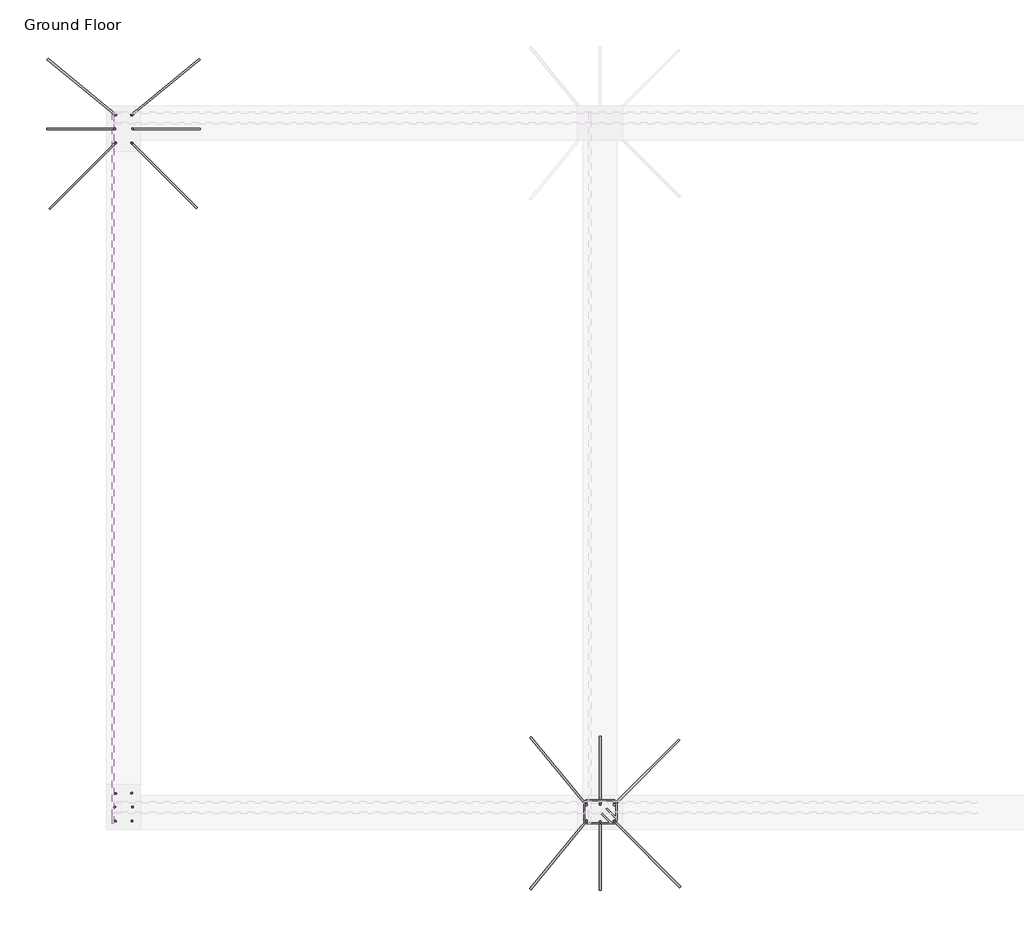
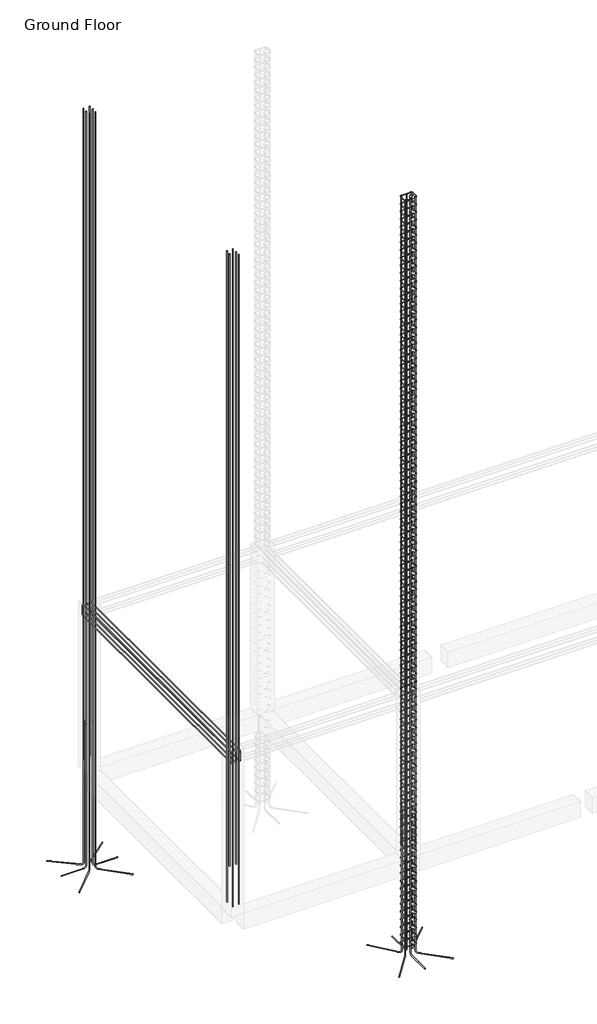
# One storey, part 2 of 5: 33 reinforcing bars.
"""IFC4 building model written with IfcOpenShell, lengths in millimetres."""

from ifc_helpers import new_model, si_unit, point, frame, origin, place, context, project, spatial, polyline, circle_curve, trimmed, segment, composite_curve, source, transform, mapped, element, save
from ifc_brep_helpers import swept_disk

model = new_model("IFC4")

# Units and contexts
model_context = context("Model", 3, world=origin())
ifc_project = project(units=[si_unit("LENGTHUNIT", "METRE", prefix="MILLI")], contexts=[model_context])

# Site, building, storey
site = spatial("IfcSite", under=ifc_project)
building = spatial("IfcBuilding", under=site)
storey = spatial("IfcBuildingStorey", under=building, Name="Ground Floor", Elevation=0.0)

# Reinforcing bars
placement = place(None, origin())
element("IfcReinforcingBar", 1, at=placement, inside=storey, context=model_context, shape_type="SolidModel", body=[
    swept_disk(composite_curve([segment(polyline([(-9208.3090827, 245.2834631, 12794.2305276), (-9208.3090827, 245.2834631, 171.0746196)]), True, "CONTINUOUS")], self_intersect=False), 6.0),
])
element("IfcReinforcingBar", 2, at=placement, inside=storey, context=model_context, shape_type="SolidModel", body=[
    swept_disk(composite_curve([segment(polyline([(-9204.3117524, 339.6230123, 888.7528218), (-9204.3117524, 339.6230123, 12792.7935546)]), True, "CONTINUOUS")], self_intersect=False), 6.0),
])
element("IfcReinforcingBar", 3, at=placement, inside=storey, context=model_context, shape_type="SolidModel", body=[
    swept_disk(composite_curve([segment(polyline([(-9210.4117524, 433.7797002, 12790.6127039), (-9210.4117524, 433.7797002, 154.6015232)]), True, "CONTINUOUS")], self_intersect=False), 6.0),
])
element("IfcReinforcingBar", 4, at=placement, inside=storey, context=model_context, shape_type="SolidModel", body=[
    swept_disk(composite_curve([segment(polyline([(-9320.9144222, 245.2834631, 12794.2305276), (-9320.9144222, 245.2834631, 159.2991411)]), True, "CONTINUOUS")], self_intersect=False), 6.0),
])
element("IfcReinforcingBar", 5, at=placement, inside=storey, context=model_context, shape_type="SolidModel", body=[
    swept_disk(composite_curve([segment(polyline([(-9324.9117524, 339.6230123, 892.2840812), (-9324.9117524, 339.6230123, 12792.7935546)]), True, "CONTINUOUS")], self_intersect=False), 6.0),
])
element("IfcReinforcingBar", 6, at=placement, inside=storey, context=model_context, shape_type="SolidModel", body=[
    swept_disk(composite_curve([segment(polyline([(-9318.8117524, 431.2797002, 12790.6127039), (-9318.8117524, 431.2797002, 134.6074908)]), True, "CONTINUOUS")], self_intersect=False), 6.0),
])
element("IfcReinforcingBar", 7, at=placement, inside=storey, context=model_context, shape_type="SolidModel", body=[
    swept_disk(composite_curve([segment(polyline([(-9208.4122575, 4816.5339681, 12794.2305276), (-9208.4122575, 4816.5339681, 171.0746196)]), True, "CONTINUOUS")], self_intersect=False), 6.0),
])
element("IfcReinforcingBar", 8, at=placement, inside=storey, context=model_context, shape_type="SolidModel", body=[
    swept_disk(composite_curve([segment(polyline([(-9204.3117524, 4911.6230123, 888.7528218), (-9204.3117524, 4911.6230123, 12792.7935546)]), True, "CONTINUOUS")], self_intersect=False), 6.0),
])
element("IfcReinforcingBar", 9, at=placement, inside=storey, context=model_context, shape_type="SolidModel", body=[
    swept_disk(composite_curve([segment(polyline([(-9208.4122575, 5005.132958, 12790.6127039), (-9208.4122575, 5005.132958, 154.6015232)]), True, "CONTINUOUS")], self_intersect=False), 6.0),
])
element("IfcReinforcingBar", 10, at=placement, inside=storey, context=model_context, shape_type="SolidModel", body=[
    swept_disk(composite_curve([segment(polyline([(-9320.8112474, 4816.5339681, 12794.2305276), (-9320.8112474, 4816.5339681, 159.2991411)]), True, "CONTINUOUS")], self_intersect=False), 6.0),
])
element("IfcReinforcingBar", 11, at=placement, inside=storey, context=model_context, shape_type="SolidModel", body=[
    swept_disk(composite_curve([segment(polyline([(-9324.9117524, 4911.6230123, 892.2840812), (-9324.9117524, 4911.6230123, 12792.7935546)]), True, "CONTINUOUS")], self_intersect=False), 6.0),
])
element("IfcReinforcingBar", 12, at=placement, inside=storey, context=model_context, shape_type="SolidModel", body=[
    swept_disk(composite_curve([segment(polyline([(-9320.8112474, 5005.132958, 12790.6127039), (-9320.8112474, 5005.132958, 134.6074908)]), True, "CONTINUOUS")], self_intersect=False), 6.0),
])
element("IfcReinforcingBar", 13, at=placement, inside=storey, context=model_context, shape_type="SolidModel", body=[
    swept_disk(composite_curve([segment(polyline([(-9209.9729913, 4816.7072019, 877.2694454), (-9209.9729913, 4816.7072019, -1868.0)]), True, "CONTINUOUS"), segment(trimmed(circle_curve(frame((-9177.4460793, 4784.1802899, -1868.0), z_axis=(-0.7071067811865491, -0.7071067811865459, 0.0), x_axis=(-32.526911999999356, 32.526911999999356, 0.0)), 46.0), [point((-9209.9729913, 4816.7072019, -1868.0))], [point((-9177.4460793, 4784.1802899, -1914.0))], True, "CARTESIAN"), True, "CONTINUOUS"), segment(polyline([(-9177.4460793, 4784.1802899, -1914.0), (-8771.7428199, 4378.4770305, -1914.0)]), True, "CONTINUOUS")], self_intersect=False), 6.0),
])
element("IfcReinforcingBar", 14, at=placement, inside=storey, context=model_context, shape_type="SolidModel", body=[
    swept_disk(composite_curve([segment(polyline([(-9318.7998971, 4817.6611074, 884.8983833), (-9318.7998971, 4817.6611074, -1868.0)]), True, "CONTINUOUS"), segment(trimmed(circle_curve(frame((-9351.326809, 4785.1341954, -1868.0), z_axis=(-0.7071067811865491, 0.707106781186546, 0.0), x_axis=(32.526911900000414, 32.526912000000266, 0.0)), 46.0), [point((-9318.7998971, 4817.6611074, -1868.0))], [point((-9351.326809, 4785.1341954, -1914.0))], True, "CARTESIAN"), True, "CONTINUOUS"), segment(polyline([(-9351.326809, 4785.1341954, -1914.0), (-9763.4563428, 4373.0046616, -1914.0)]), True, "CONTINUOUS")], self_intersect=False), 6.0),
])
element("IfcReinforcingBar", 15, at=placement, inside=storey, context=model_context, shape_type="SolidModel", body=[
    swept_disk(composite_curve([segment(polyline([(-9211.2828277, 5004.9867911, 871.8711989), (-9211.2828277, 5004.9867911, -1868.0)]), True, "CONTINUOUS"), segment(trimmed(circle_curve(frame((-9175.7367573, 5034.1839978, -1868.0), z_axis=(0.634721884628903, -0.7727406610067401, 0.0), x_axis=(-35.546070400001554, -29.197206699999697, 0.0)), 46.0), [point((-9211.2828277, 5004.9867911, -1868.0))], [point((-9175.7367573, 5034.1839978, -1914.0))], True, "CARTESIAN"), True, "CONTINUOUS"), segment(polyline([(-9175.7367573, 5034.1839978, -1914.0), (-8753.4008173, 5381.0867522, -1914.0)]), True, "CONTINUOUS")], self_intersect=False), 6.0),
])
element("IfcReinforcingBar", 16, at=placement, inside=storey, context=model_context, shape_type="SolidModel", body=[
    swept_disk(composite_curve([segment(polyline([(-9317.9839747, 5004.7322479, 890.3940928), (-9317.9839747, 5004.7322479, -1868.0)]), True, "CONTINUOUS"), segment(trimmed(circle_curve(frame((-9353.5300451, 5033.9294546, -1868.0), z_axis=(0.6347218846289031, 0.7727406610067401, 0.0), x_axis=(35.546070399999735, -29.197206699999697, 0.0)), 46.0), [point((-9317.9839747, 5004.7322479, -1868.0))], [point((-9353.5300451, 5033.9294546, -1914.0))], True, "CARTESIAN"), True, "CONTINUOUS"), segment(polyline([(-9353.5300451, 5033.9294546, -1914.0), (-9777.6976875, 5382.3367522, -1914.0)]), True, "CONTINUOUS")], self_intersect=False), 6.0),
])
element("IfcReinforcingBar", 17, at=placement, inside=storey, context=model_context, shape_type="SolidModel", body=[
    swept_disk(composite_curve([segment(polyline([(-9204.3117524, 4911.6230123, 875.7528218), (-9204.3117524, 4911.6230123, -1868.0)]), True, "CONTINUOUS"), segment(trimmed(circle_curve(frame((-9158.3117524, 4911.6230123, -1868.0), z_axis=(0.0, -1.0, 0.0), x_axis=(-46.0, 0.0, 0.0)), 46.0), [point((-9204.3117524, 4911.6230123, -1868.0))], [point((-9158.3117524, 4911.6230123, -1914.0))], True, "CARTESIAN"), True, "CONTINUOUS"), segment(polyline([(-9158.3117524, 4911.6230123, -1914.0), (-8747.3359391, 4911.6230123, -1914.0)]), True, "CONTINUOUS")], self_intersect=False), 6.0),
])
element("IfcReinforcingBar", 18, at=placement, inside=storey, context=model_context, shape_type="SolidModel", body=[
    swept_disk(composite_curve([segment(polyline([(-9324.9117524, 4911.6230123, 879.2840812), (-9324.9117524, 4911.6230123, -1868.0)]), True, "CONTINUOUS"), segment(trimmed(circle_curve(frame((-9370.9117524, 4911.6230123, -1868.0), z_axis=(0.0, 1.0, 0.0), x_axis=(46.0, 0.0, 0.0)), 46.0), [point((-9324.9117524, 4911.6230123, -1868.0))], [point((-9370.9117524, 4911.6230123, -1914.0))], True, "CARTESIAN"), True, "CONTINUOUS"), segment(polyline([(-9370.9117524, 4911.6230123, -1914.0), (-9784.4222077, 4911.6230123, -1914.0)]), True, "CONTINUOUS")], self_intersect=False), 6.0),
])
element("IfcReinforcingBar", 19, at=placement, inside=storey, context=model_context, shape_type="SolidModel", body=[
    swept_disk(composite_curve([segment(polyline([(-5957.3854913, 355.3722242, 877.2694454), (-5957.3854913, 355.3722242, -1868.0)]), True, "CONTINUOUS"), segment(trimmed(circle_curve(frame((-5924.8585793, 387.8991362, -1868.0), z_axis=(0.7071067811865447, -0.7071067811865503, 0.0), x_axis=(-32.526911999999356, -32.52691199999998, 0.0)), 46.0), [point((-5957.3854913, 355.3722242, -1868.0))], [point((-5924.8585793, 387.8991362, -1914.0))], True, "CARTESIAN"), True, "CONTINUOUS"), segment(polyline([(-5924.8585793, 387.8991362, -1914.0), (-5519.1553199, 793.6023956, -1914.0)]), True, "CONTINUOUS")], self_intersect=False), 6.0),
])
element("IfcReinforcingBar", 20, at=placement, inside=storey, context=model_context, shape_type="SolidModel", body=[
    swept_disk(composite_curve([segment(polyline([(-5958.3393967, 246.5453184, 884.8983833), (-5958.3393967, 246.5453184, -1868.0)]), True, "CONTINUOUS"), segment(trimmed(circle_curve(frame((-5925.8124848, 214.0184065, -1868.0), z_axis=(-0.7071067811865472, -0.7071067811865479, 0.0), x_axis=(-32.526911900000414, 32.526911900000016, 0.0)), 46.0), [point((-5958.3393967, 246.5453184, -1868.0))], [point((-5925.8124848, 214.0184065, -1914.0))], True, "CARTESIAN"), True, "CONTINUOUS"), segment(polyline([(-5925.8124848, 214.0184065, -1914.0), (-5513.682951, -198.1111273, -1914.0)]), True, "CONTINUOUS")], self_intersect=False), 6.0),
])
element("IfcReinforcingBar", 21, at=placement, inside=storey, context=model_context, shape_type="SolidModel", body=[
    swept_disk(composite_curve([segment(polyline([(-6145.6650805, 354.0623878, 871.8711989), (-6145.6650805, 354.0623878, -1868.0)]), True, "CONTINUOUS"), segment(trimmed(circle_curve(frame((-6174.8622872, 389.6084582, -1868.0), z_axis=(0.7727406610067412, 0.6347218846289017, 0.0), x_axis=(29.197206699999697, -35.54607039999996, 0.0)), 46.0), [point((-6145.6650805, 354.0623878, -1868.0))], [point((-6174.8622872, 389.6084582, -1914.0))], True, "CARTESIAN"), True, "CONTINUOUS"), segment(polyline([(-6174.8622872, 389.6084582, -1914.0), (-6521.7650416, 811.9443982, -1914.0)]), True, "CONTINUOUS")], self_intersect=False), 6.0),
])
element("IfcReinforcingBar", 22, at=placement, inside=storey, context=model_context, shape_type="SolidModel", body=[
    swept_disk(composite_curve([segment(polyline([(-6145.4105373, 247.3612408, 890.3940928), (-6145.4105373, 247.3612408, -1868.0)]), True, "CONTINUOUS"), segment(trimmed(circle_curve(frame((-6174.607744, 211.8151704, -1868.0), z_axis=(-0.7727406610067391, 0.6347218846289043, 0.0), x_axis=(29.197206699999697, 35.54607039999999, 0.0)), 46.0), [point((-6145.4105373, 247.3612408, -1868.0))], [point((-6174.607744, 211.8151704, -1914.0))], True, "CARTESIAN"), True, "CONTINUOUS"), segment(polyline([(-6174.607744, 211.8151704, -1914.0), (-6523.0150416, -212.3524721, -1914.0)]), True, "CONTINUOUS")], self_intersect=False), 6.0),
])
element("IfcReinforcingBar", 23, at=placement, inside=storey, context=model_context, shape_type="SolidModel", body=[
    swept_disk(composite_curve([segment(polyline([(-6052.3013017, 359.1834631, 875.7528218), (-6052.3013017, 359.1834631, -1868.0)]), True, "CONTINUOUS"), segment(trimmed(circle_curve(frame((-6052.3013017, 405.1834631, -1868.0), z_axis=(1.0, 0.0, 0.0), x_axis=(0.0, -46.0, 0.0)), 46.0), [point((-6052.3013017, 359.1834631, -1868.0))], [point((-6052.3013017, 405.1834631, -1914.0))], True, "CARTESIAN"), True, "CONTINUOUS"), segment(polyline([(-6052.3013017, 405.1834631, -1914.0), (-6052.3013017, 818.0092764, -1914.0)]), True, "CONTINUOUS")], self_intersect=False), 6.0),
])
element("IfcReinforcingBar", 24, at=placement, inside=storey, context=model_context, shape_type="SolidModel", body=[
    swept_disk(composite_curve([segment(polyline([(-6052.3013017, 240.4334631, 879.2840812), (-6052.3013017, 240.4334631, -1868.0)]), True, "CONTINUOUS"), segment(trimmed(circle_curve(frame((-6052.3013017, 194.4334631, -1868.0), z_axis=(-1.0, 0.0, 0.0), x_axis=(0.0, 46.0, 0.0)), 46.0), [point((-6052.3013017, 240.4334631, -1868.0))], [point((-6052.3013017, 194.4334631, -1914.0))], True, "CARTESIAN"), True, "CONTINUOUS"), segment(polyline([(-6052.3013017, 194.4334631, -1914.0), (-6052.3013017, -219.0769922, -1914.0)]), True, "CONTINUOUS")], self_intersect=False), 6.0),
])
reinforcing_bar_shape = source(origin(), model_context, "Body", "SolidModel", [
    swept_disk(composite_curve([segment(polyline([(-6041.6771046, 295.0576897, -1724.0), (-5984.0823152, 237.4629003, -1724.0)]), True, "CONTINUOUS"), segment(trimmed(circle_curve(frame((-5967.1117524, 254.4334631, -1724.0), z_axis=(0.0, 0.0, 1.0), x_axis=(-16.970562800000152, -16.97056280000001, 0.0)), 24.0), [point((-5984.0823152, 237.4629003, -1724.0))], [point((-5943.1117524, 254.4334631, -1724.0))], True, "CARTESIAN"), True, "CONTINUOUS"), segment(polyline([(-5943.1117524, 254.4334631, -1724.0), (-5943.1117524, 362.0334631, -1724.0)]), True, "CONTINUOUS"), segment(trimmed(circle_curve(frame((-5967.1117524, 362.0334631, -1724.0), z_axis=(0.0, 0.0, 1.0), x_axis=(24.0, 0.0, 0.0)), 24.0), [point((-5943.1117524, 362.0334631, -1724.0))], [point((-5967.1117524, 386.0334631, -1724.0))], True, "CARTESIAN"), True, "CONTINUOUS"), segment(polyline([(-5967.1117524, 386.0334631, -1724.0), (-6135.9117524, 386.0334631, -1724.0)]), True, "CONTINUOUS"), segment(trimmed(circle_curve(frame((-6135.9117524, 362.0651209, -1725.2323055), z_axis=(0.0, -0.05134606277296417, 0.9986809209340664), x_axis=(0.0, 23.968342199999995, 1.2323054999999385)), 24.0), [point((-6135.9117524, 386.0334631, -1724.0))], [point((-6159.9117524, 362.0651209, -1725.2323055))], True, "CARTESIAN"), True, "CONTINUOUS"), segment(polyline([(-6159.9117524, 362.0651209, -1725.2323055), (-6159.9117524, 254.4018052, -1730.7676945)]), True, "CONTINUOUS"), segment(trimmed(circle_curve(frame((-6135.9117524, 254.4018052, -1730.7676945), z_axis=(0.0, -0.05134606277296417, 0.9986809209340664), x_axis=(-24.0, 0.0, 0.0)), 24.0), [point((-6159.9117524, 254.4018052, -1730.7676945))], [point((-6135.9117524, 230.4334631, -1732.0))], True, "CARTESIAN"), True, "CONTINUOUS"), segment(polyline([(-6135.9117524, 230.4334631, -1732.0), (-5967.1117524, 230.4334631, -1732.0)]), True, "CONTINUOUS"), segment(trimmed(circle_curve(frame((-5967.1117524, 254.4334631, -1732.0), z_axis=(0.0, 0.0, 1.0), x_axis=(0.0, -24.0, 0.0)), 24.0), [point((-5967.1117524, 230.4334631, -1732.0))], [point((-5950.1411897, 271.4040258, -1732.0))], True, "CARTESIAN"), True, "CONTINUOUS"), segment(polyline([(-5950.1411897, 271.4040258, -1732.0), (-6007.7359791, 328.9988152, -1732.0)]), True, "CONTINUOUS")], self_intersect=False), 4.0),
])
element("IfcReinforcingBar", 25, at=placement, inside=storey, context=model_context, shape_type="MappedRepresentation", body=[
    mapped(reinforcing_bar_shape, transform((0.0, 0.0, 0.0), x_axis=(1.0, 0.0, 0.0), y_axis=(0.0, 1.0, 0.0), z_axis=(0.0, 0.0, 1.0))),
    mapped(reinforcing_bar_shape, transform((0.0, 0.0, 149.5904239), x_axis=(1.0, 0.0, 0.0), y_axis=(0.0, 1.0, 0.0), z_axis=(0.0, 0.0, 1.0))),
    mapped(reinforcing_bar_shape, transform((0.0, 0.0, 299.1808479), x_axis=(1.0, 0.0, 0.0), y_axis=(0.0, 1.0, 0.0), z_axis=(0.0, 0.0, 1.0))),
    mapped(reinforcing_bar_shape, transform((0.0, 0.0, 448.7712718), x_axis=(1.0, 0.0, 0.0), y_axis=(0.0, 1.0, 0.0), z_axis=(0.0, 0.0, 1.0))),
    mapped(reinforcing_bar_shape, transform((0.0, 0.0, 598.3616957), x_axis=(1.0, 0.0, 0.0), y_axis=(0.0, 1.0, 0.0), z_axis=(0.0, 0.0, 1.0))),
    mapped(reinforcing_bar_shape, transform((0.0, 0.0, 747.9521197), x_axis=(1.0, 0.0, 0.0), y_axis=(0.0, 1.0, 0.0), z_axis=(0.0, 0.0, 1.0))),
    mapped(reinforcing_bar_shape, transform((0.0, 0.0, 897.5425436), x_axis=(1.0, 0.0, 0.0), y_axis=(0.0, 1.0, 0.0), z_axis=(0.0, 0.0, 1.0))),
    mapped(reinforcing_bar_shape, transform((0.0, 0.0, 1047.1329675), x_axis=(1.0, 0.0, 0.0), y_axis=(0.0, 1.0, 0.0), z_axis=(0.0, 0.0, 1.0))),
    mapped(reinforcing_bar_shape, transform((0.0, 0.0, 1196.7233914), x_axis=(1.0, 0.0, 0.0), y_axis=(0.0, 1.0, 0.0), z_axis=(0.0, 0.0, 1.0))),
    mapped(reinforcing_bar_shape, transform((0.0, 0.0, 1346.3138154), x_axis=(1.0, 0.0, 0.0), y_axis=(0.0, 1.0, 0.0), z_axis=(0.0, 0.0, 1.0))),
    mapped(reinforcing_bar_shape, transform((0.0, 0.0, 1495.9042393), x_axis=(1.0, 0.0, 0.0), y_axis=(0.0, 1.0, 0.0), z_axis=(0.0, 0.0, 1.0))),
    mapped(reinforcing_bar_shape, transform((0.0, 0.0, 1645.4946632), x_axis=(1.0, 0.0, 0.0), y_axis=(0.0, 1.0, 0.0), z_axis=(0.0, 0.0, 1.0))),
    mapped(reinforcing_bar_shape, transform((0.0, 0.0, 1795.0850872), x_axis=(1.0, 0.0, 0.0), y_axis=(0.0, 1.0, 0.0), z_axis=(0.0, 0.0, 1.0))),
    mapped(reinforcing_bar_shape, transform((0.0, 0.0, 1944.6755111), x_axis=(1.0, 0.0, 0.0), y_axis=(0.0, 1.0, 0.0), z_axis=(0.0, 0.0, 1.0))),
    mapped(reinforcing_bar_shape, transform((0.0, 0.0, 2094.265935), x_axis=(1.0, 0.0, 0.0), y_axis=(0.0, 1.0, 0.0), z_axis=(0.0, 0.0, 1.0))),
    mapped(reinforcing_bar_shape, transform((0.0, 0.0, 2243.856359), x_axis=(1.0, 0.0, 0.0), y_axis=(0.0, 1.0, 0.0), z_axis=(0.0, 0.0, 1.0))),
    mapped(reinforcing_bar_shape, transform((0.0, 0.0, 2393.4467829), x_axis=(1.0, 0.0, 0.0), y_axis=(0.0, 1.0, 0.0), z_axis=(0.0, 0.0, 1.0))),
    mapped(reinforcing_bar_shape, transform((0.0, 0.0, 2543.0372068), x_axis=(1.0, 0.0, 0.0), y_axis=(0.0, 1.0, 0.0), z_axis=(0.0, 0.0, 1.0))),
    mapped(reinforcing_bar_shape, transform((0.0, 0.0, 2692.6276307), x_axis=(1.0, 0.0, 0.0), y_axis=(0.0, 1.0, 0.0), z_axis=(0.0, 0.0, 1.0))),
    mapped(reinforcing_bar_shape, transform((0.0, 0.0, 2842.2180547), x_axis=(1.0, 0.0, 0.0), y_axis=(0.0, 1.0, 0.0), z_axis=(0.0, 0.0, 1.0))),
    mapped(reinforcing_bar_shape, transform((0.0, 0.0, 2991.8084786), x_axis=(1.0, 0.0, 0.0), y_axis=(0.0, 1.0, 0.0), z_axis=(0.0, 0.0, 1.0))),
    mapped(reinforcing_bar_shape, transform((0.0, 0.0, 3141.3989025), x_axis=(1.0, 0.0, 0.0), y_axis=(0.0, 1.0, 0.0), z_axis=(0.0, 0.0, 1.0))),
    mapped(reinforcing_bar_shape, transform((0.0, 0.0, 3290.9893265), x_axis=(1.0, 0.0, 0.0), y_axis=(0.0, 1.0, 0.0), z_axis=(0.0, 0.0, 1.0))),
    mapped(reinforcing_bar_shape, transform((0.0, 0.0, 3440.5797504), x_axis=(1.0, 0.0, 0.0), y_axis=(0.0, 1.0, 0.0), z_axis=(0.0, 0.0, 1.0))),
    mapped(reinforcing_bar_shape, transform((0.0, 0.0, 3590.1701743), x_axis=(1.0, 0.0, 0.0), y_axis=(0.0, 1.0, 0.0), z_axis=(0.0, 0.0, 1.0))),
    mapped(reinforcing_bar_shape, transform((0.0, 0.0, 3739.7605983), x_axis=(1.0, 0.0, 0.0), y_axis=(0.0, 1.0, 0.0), z_axis=(0.0, 0.0, 1.0))),
    mapped(reinforcing_bar_shape, transform((0.0, 0.0, 3889.3510222), x_axis=(1.0, 0.0, 0.0), y_axis=(0.0, 1.0, 0.0), z_axis=(0.0, 0.0, 1.0))),
    mapped(reinforcing_bar_shape, transform((0.0, 0.0, 4038.9414461), x_axis=(1.0, 0.0, 0.0), y_axis=(0.0, 1.0, 0.0), z_axis=(0.0, 0.0, 1.0))),
    mapped(reinforcing_bar_shape, transform((0.0, 0.0, 4188.53187), x_axis=(1.0, 0.0, 0.0), y_axis=(0.0, 1.0, 0.0), z_axis=(0.0, 0.0, 1.0))),
    mapped(reinforcing_bar_shape, transform((0.0, 0.0, 4338.122294), x_axis=(1.0, 0.0, 0.0), y_axis=(0.0, 1.0, 0.0), z_axis=(0.0, 0.0, 1.0))),
    mapped(reinforcing_bar_shape, transform((0.0, 0.0, 4487.7127179), x_axis=(1.0, 0.0, 0.0), y_axis=(0.0, 1.0, 0.0), z_axis=(0.0, 0.0, 1.0))),
    mapped(reinforcing_bar_shape, transform((0.0, 0.0, 4637.3031418), x_axis=(1.0, 0.0, 0.0), y_axis=(0.0, 1.0, 0.0), z_axis=(0.0, 0.0, 1.0))),
    mapped(reinforcing_bar_shape, transform((0.0, 0.0, 4786.8935658), x_axis=(1.0, 0.0, 0.0), y_axis=(0.0, 1.0, 0.0), z_axis=(0.0, 0.0, 1.0))),
    mapped(reinforcing_bar_shape, transform((0.0, 0.0, 4936.4839897), x_axis=(1.0, 0.0, 0.0), y_axis=(0.0, 1.0, 0.0), z_axis=(0.0, 0.0, 1.0))),
    mapped(reinforcing_bar_shape, transform((0.0, 0.0, 5086.0744136), x_axis=(1.0, 0.0, 0.0), y_axis=(0.0, 1.0, 0.0), z_axis=(0.0, 0.0, 1.0))),
    mapped(reinforcing_bar_shape, transform((0.0, 0.0, 5235.6648376), x_axis=(1.0, 0.0, 0.0), y_axis=(0.0, 1.0, 0.0), z_axis=(0.0, 0.0, 1.0))),
    mapped(reinforcing_bar_shape, transform((0.0, 0.0, 5385.2552615), x_axis=(1.0, 0.0, 0.0), y_axis=(0.0, 1.0, 0.0), z_axis=(0.0, 0.0, 1.0))),
    mapped(reinforcing_bar_shape, transform((0.0, 0.0, 5534.8456854), x_axis=(1.0, 0.0, 0.0), y_axis=(0.0, 1.0, 0.0), z_axis=(0.0, 0.0, 1.0))),
    mapped(reinforcing_bar_shape, transform((0.0, 0.0, 5684.4361094), x_axis=(1.0, 0.0, 0.0), y_axis=(0.0, 1.0, 0.0), z_axis=(0.0, 0.0, 1.0))),
    mapped(reinforcing_bar_shape, transform((0.0, 0.0, 5834.0265333), x_axis=(1.0, 0.0, 0.0), y_axis=(0.0, 1.0, 0.0), z_axis=(0.0, 0.0, 1.0))),
    mapped(reinforcing_bar_shape, transform((0.0, 0.0, 5983.6169572), x_axis=(1.0, 0.0, 0.0), y_axis=(0.0, 1.0, 0.0), z_axis=(0.0, 0.0, 1.0))),
    mapped(reinforcing_bar_shape, transform((0.0, 0.0, 6133.2073811), x_axis=(1.0, 0.0, 0.0), y_axis=(0.0, 1.0, 0.0), z_axis=(0.0, 0.0, 1.0))),
    mapped(reinforcing_bar_shape, transform((0.0, 0.0, 6282.7978051), x_axis=(1.0, 0.0, 0.0), y_axis=(0.0, 1.0, 0.0), z_axis=(0.0, 0.0, 1.0))),
    mapped(reinforcing_bar_shape, transform((0.0, 0.0, 6432.388229), x_axis=(1.0, 0.0, 0.0), y_axis=(0.0, 1.0, 0.0), z_axis=(0.0, 0.0, 1.0))),
    mapped(reinforcing_bar_shape, transform((0.0, 0.0, 6581.9786529), x_axis=(1.0, 0.0, 0.0), y_axis=(0.0, 1.0, 0.0), z_axis=(0.0, 0.0, 1.0))),
    mapped(reinforcing_bar_shape, transform((0.0, 0.0, 6731.5690769), x_axis=(1.0, 0.0, 0.0), y_axis=(0.0, 1.0, 0.0), z_axis=(0.0, 0.0, 1.0))),
    mapped(reinforcing_bar_shape, transform((0.0, 0.0, 6881.1595008), x_axis=(1.0, 0.0, 0.0), y_axis=(0.0, 1.0, 0.0), z_axis=(0.0, 0.0, 1.0))),
    mapped(reinforcing_bar_shape, transform((0.0, 0.0, 7030.7499247), x_axis=(1.0, 0.0, 0.0), y_axis=(0.0, 1.0, 0.0), z_axis=(0.0, 0.0, 1.0))),
    mapped(reinforcing_bar_shape, transform((0.0, 0.0, 7180.3403487), x_axis=(1.0, 0.0, 0.0), y_axis=(0.0, 1.0, 0.0), z_axis=(0.0, 0.0, 1.0))),
    mapped(reinforcing_bar_shape, transform((0.0, 0.0, 7329.9307726), x_axis=(1.0, 0.0, 0.0), y_axis=(0.0, 1.0, 0.0), z_axis=(0.0, 0.0, 1.0))),
    mapped(reinforcing_bar_shape, transform((0.0, 0.0, 7479.5211965), x_axis=(1.0, 0.0, 0.0), y_axis=(0.0, 1.0, 0.0), z_axis=(0.0, 0.0, 1.0))),
    mapped(reinforcing_bar_shape, transform((0.0, 0.0, 7629.1116204), x_axis=(1.0, 0.0, 0.0), y_axis=(0.0, 1.0, 0.0), z_axis=(0.0, 0.0, 1.0))),
    mapped(reinforcing_bar_shape, transform((0.0, 0.0, 7778.7020444), x_axis=(1.0, 0.0, 0.0), y_axis=(0.0, 1.0, 0.0), z_axis=(0.0, 0.0, 1.0))),
    mapped(reinforcing_bar_shape, transform((0.0, 0.0, 7928.2924683), x_axis=(1.0, 0.0, 0.0), y_axis=(0.0, 1.0, 0.0), z_axis=(0.0, 0.0, 1.0))),
    mapped(reinforcing_bar_shape, transform((0.0, 0.0, 8077.8828922), x_axis=(1.0, 0.0, 0.0), y_axis=(0.0, 1.0, 0.0), z_axis=(0.0, 0.0, 1.0))),
    mapped(reinforcing_bar_shape, transform((0.0, 0.0, 8227.4733162), x_axis=(1.0, 0.0, 0.0), y_axis=(0.0, 1.0, 0.0), z_axis=(0.0, 0.0, 1.0))),
    mapped(reinforcing_bar_shape, transform((0.0, 0.0, 8377.0637401), x_axis=(1.0, 0.0, 0.0), y_axis=(0.0, 1.0, 0.0), z_axis=(0.0, 0.0, 1.0))),
    mapped(reinforcing_bar_shape, transform((0.0, 0.0, 8526.654164), x_axis=(1.0, 0.0, 0.0), y_axis=(0.0, 1.0, 0.0), z_axis=(0.0, 0.0, 1.0))),
    mapped(reinforcing_bar_shape, transform((0.0, 0.0, 8676.244588), x_axis=(1.0, 0.0, 0.0), y_axis=(0.0, 1.0, 0.0), z_axis=(0.0, 0.0, 1.0))),
    mapped(reinforcing_bar_shape, transform((0.0, 0.0, 8825.8350119), x_axis=(1.0, 0.0, 0.0), y_axis=(0.0, 1.0, 0.0), z_axis=(0.0, 0.0, 1.0))),
    mapped(reinforcing_bar_shape, transform((0.0, 0.0, 8975.4254358), x_axis=(1.0, 0.0, 0.0), y_axis=(0.0, 1.0, 0.0), z_axis=(0.0, 0.0, 1.0))),
    mapped(reinforcing_bar_shape, transform((0.0, 0.0, 9125.0158597), x_axis=(1.0, 0.0, 0.0), y_axis=(0.0, 1.0, 0.0), z_axis=(0.0, 0.0, 1.0))),
    mapped(reinforcing_bar_shape, transform((0.0, 0.0, 9274.6062837), x_axis=(1.0, 0.0, 0.0), y_axis=(0.0, 1.0, 0.0), z_axis=(0.0, 0.0, 1.0))),
    mapped(reinforcing_bar_shape, transform((0.0, 0.0, 9424.1967076), x_axis=(1.0, 0.0, 0.0), y_axis=(0.0, 1.0, 0.0), z_axis=(0.0, 0.0, 1.0))),
    mapped(reinforcing_bar_shape, transform((0.0, 0.0, 9573.7871315), x_axis=(1.0, 0.0, 0.0), y_axis=(0.0, 1.0, 0.0), z_axis=(0.0, 0.0, 1.0))),
    mapped(reinforcing_bar_shape, transform((0.0, 0.0, 9723.3775555), x_axis=(1.0, 0.0, 0.0), y_axis=(0.0, 1.0, 0.0), z_axis=(0.0, 0.0, 1.0))),
    mapped(reinforcing_bar_shape, transform((0.0, 0.0, 9872.9679794), x_axis=(1.0, 0.0, 0.0), y_axis=(0.0, 1.0, 0.0), z_axis=(0.0, 0.0, 1.0))),
    mapped(reinforcing_bar_shape, transform((0.0, 0.0, 10022.5584033), x_axis=(1.0, 0.0, 0.0), y_axis=(0.0, 1.0, 0.0), z_axis=(0.0, 0.0, 1.0))),
    mapped(reinforcing_bar_shape, transform((0.0, 0.0, 10172.1488273), x_axis=(1.0, 0.0, 0.0), y_axis=(0.0, 1.0, 0.0), z_axis=(0.0, 0.0, 1.0))),
    mapped(reinforcing_bar_shape, transform((0.0, 0.0, 10321.7392512), x_axis=(1.0, 0.0, 0.0), y_axis=(0.0, 1.0, 0.0), z_axis=(0.0, 0.0, 1.0))),
    mapped(reinforcing_bar_shape, transform((0.0, 0.0, 10471.3296751), x_axis=(1.0, 0.0, 0.0), y_axis=(0.0, 1.0, 0.0), z_axis=(0.0, 0.0, 1.0))),
    mapped(reinforcing_bar_shape, transform((0.0, 0.0, 10620.9200991), x_axis=(1.0, 0.0, 0.0), y_axis=(0.0, 1.0, 0.0), z_axis=(0.0, 0.0, 1.0))),
    mapped(reinforcing_bar_shape, transform((0.0, 0.0, 10770.510523), x_axis=(1.0, 0.0, 0.0), y_axis=(0.0, 1.0, 0.0), z_axis=(0.0, 0.0, 1.0))),
    mapped(reinforcing_bar_shape, transform((0.0, 0.0, 10920.1009469), x_axis=(1.0, 0.0, 0.0), y_axis=(0.0, 1.0, 0.0), z_axis=(0.0, 0.0, 1.0))),
    mapped(reinforcing_bar_shape, transform((0.0, 0.0, 11069.6913708), x_axis=(1.0, 0.0, 0.0), y_axis=(0.0, 1.0, 0.0), z_axis=(0.0, 0.0, 1.0))),
    mapped(reinforcing_bar_shape, transform((0.0, 0.0, 11219.2817948), x_axis=(1.0, 0.0, 0.0), y_axis=(0.0, 1.0, 0.0), z_axis=(0.0, 0.0, 1.0))),
    mapped(reinforcing_bar_shape, transform((0.0, 0.0, 11368.8722187), x_axis=(1.0, 0.0, 0.0), y_axis=(0.0, 1.0, 0.0), z_axis=(0.0, 0.0, 1.0))),
    mapped(reinforcing_bar_shape, transform((0.0, 0.0, 11518.4626426), x_axis=(1.0, 0.0, 0.0), y_axis=(0.0, 1.0, 0.0), z_axis=(0.0, 0.0, 1.0))),
    mapped(reinforcing_bar_shape, transform((0.0, 0.0, 11668.0530666), x_axis=(1.0, 0.0, 0.0), y_axis=(0.0, 1.0, 0.0), z_axis=(0.0, 0.0, 1.0))),
    mapped(reinforcing_bar_shape, transform((0.0, 0.0, 11817.6434905), x_axis=(1.0, 0.0, 0.0), y_axis=(0.0, 1.0, 0.0), z_axis=(0.0, 0.0, 1.0))),
    mapped(reinforcing_bar_shape, transform((0.0, 0.0, 11967.2339144), x_axis=(1.0, 0.0, 0.0), y_axis=(0.0, 1.0, 0.0), z_axis=(0.0, 0.0, 1.0))),
    mapped(reinforcing_bar_shape, transform((0.0, 0.0, 12116.8243384), x_axis=(1.0, 0.0, 0.0), y_axis=(0.0, 1.0, 0.0), z_axis=(0.0, 0.0, 1.0))),
    mapped(reinforcing_bar_shape, transform((0.0, 0.0, 12266.4147623), x_axis=(1.0, 0.0, 0.0), y_axis=(0.0, 1.0, 0.0), z_axis=(0.0, 0.0, 1.0))),
    mapped(reinforcing_bar_shape, transform((0.0, 0.0, 12416.0051862), x_axis=(1.0, 0.0, 0.0), y_axis=(0.0, 1.0, 0.0), z_axis=(0.0, 0.0, 1.0))),
    mapped(reinforcing_bar_shape, transform((0.0, 0.0, 12565.5956101), x_axis=(1.0, 0.0, 0.0), y_axis=(0.0, 1.0, 0.0), z_axis=(0.0, 0.0, 1.0))),
    mapped(reinforcing_bar_shape, transform((0.0, 0.0, 12715.1860341), x_axis=(1.0, 0.0, 0.0), y_axis=(0.0, 1.0, 0.0), z_axis=(0.0, 0.0, 1.0))),
    mapped(reinforcing_bar_shape, transform((0.0, 0.0, 12864.776458), x_axis=(1.0, 0.0, 0.0), y_axis=(0.0, 1.0, 0.0), z_axis=(0.0, 0.0, 1.0))),
    mapped(reinforcing_bar_shape, transform((0.0, 0.0, 13014.3668819), x_axis=(1.0, 0.0, 0.0), y_axis=(0.0, 1.0, 0.0), z_axis=(0.0, 0.0, 1.0))),
    mapped(reinforcing_bar_shape, transform((0.0, 0.0, 13163.9573059), x_axis=(1.0, 0.0, 0.0), y_axis=(0.0, 1.0, 0.0), z_axis=(0.0, 0.0, 1.0))),
    mapped(reinforcing_bar_shape, transform((0.0, 0.0, 13313.5477298), x_axis=(1.0, 0.0, 0.0), y_axis=(0.0, 1.0, 0.0), z_axis=(0.0, 0.0, 1.0))),
    mapped(reinforcing_bar_shape, transform((0.0, 0.0, 13463.1381537), x_axis=(1.0, 0.0, 0.0), y_axis=(0.0, 1.0, 0.0), z_axis=(0.0, 0.0, 1.0))),
    mapped(reinforcing_bar_shape, transform((0.0, 0.0, 13612.7285777), x_axis=(1.0, 0.0, 0.0), y_axis=(0.0, 1.0, 0.0), z_axis=(0.0, 0.0, 1.0))),
    mapped(reinforcing_bar_shape, transform((0.0, 0.0, 13762.3190016), x_axis=(1.0, 0.0, 0.0), y_axis=(0.0, 1.0, 0.0), z_axis=(0.0, 0.0, 1.0))),
    mapped(reinforcing_bar_shape, transform((0.0, 0.0, 13911.9094255), x_axis=(1.0, 0.0, 0.0), y_axis=(0.0, 1.0, 0.0), z_axis=(0.0, 0.0, 1.0))),
    mapped(reinforcing_bar_shape, transform((0.0, 0.0, 14061.4998494), x_axis=(1.0, 0.0, 0.0), y_axis=(0.0, 1.0, 0.0), z_axis=(0.0, 0.0, 1.0))),
    mapped(reinforcing_bar_shape, transform((0.0, 0.0, 14211.0902734), x_axis=(1.0, 0.0, 0.0), y_axis=(0.0, 1.0, 0.0), z_axis=(0.0, 0.0, 1.0))),
    mapped(reinforcing_bar_shape, transform((0.0, 0.0, 14360.6806973), x_axis=(1.0, 0.0, 0.0), y_axis=(0.0, 1.0, 0.0), z_axis=(0.0, 0.0, 1.0))),
    mapped(reinforcing_bar_shape, transform((0.0, 0.0, 14510.2711212), x_axis=(1.0, 0.0, 0.0), y_axis=(0.0, 1.0, 0.0), z_axis=(0.0, 0.0, 1.0))),
])
element("IfcReinforcingBar", 26, at=placement, inside=storey, context=model_context, shape_type="SolidModel", body=[
    swept_disk(composite_curve([segment(polyline([(-5957.2122575, 371.932958, 12794.2305276), (-5957.2122575, 371.932958, 171.0746196)]), True, "CONTINUOUS")], self_intersect=False), 6.0),
])
element("IfcReinforcingBar", 27, at=placement, inside=storey, context=model_context, shape_type="SolidModel", body=[
    swept_disk(composite_curve([segment(polyline([(-6052.3013017, 359.1834631, 888.7528218), (-6052.3013017, 359.1834631, 12792.7935546)]), True, "CONTINUOUS")], self_intersect=False), 6.0),
])
element("IfcReinforcingBar", 28, at=placement, inside=storey, context=model_context, shape_type="SolidModel", body=[
    swept_disk(composite_curve([segment(polyline([(-6145.8112474, 371.932958, 12790.6127039), (-6145.8112474, 371.932958, 154.6015232)]), True, "CONTINUOUS")], self_intersect=False), 6.0),
])
element("IfcReinforcingBar", 29, at=placement, inside=storey, context=model_context, shape_type="SolidModel", body=[
    swept_disk(composite_curve([segment(polyline([(-5957.2122575, 244.5339681, 12794.2305276), (-5957.2122575, 244.5339681, 159.2991411)]), True, "CONTINUOUS")], self_intersect=False), 6.0),
])
element("IfcReinforcingBar", 30, at=placement, inside=storey, context=model_context, shape_type="SolidModel", body=[
    swept_disk(composite_curve([segment(polyline([(-6052.3013017, 240.4334631, 892.2840812), (-6052.3013017, 240.4334631, 12792.7935546)]), True, "CONTINUOUS")], self_intersect=False), 6.0),
])
element("IfcReinforcingBar", 31, at=placement, inside=storey, context=model_context, shape_type="SolidModel", body=[
    swept_disk(composite_curve([segment(polyline([(-6145.8112474, 244.5339681, 12790.6127039), (-6145.8112474, 244.5339681, 134.6074908)]), True, "CONTINUOUS")], self_intersect=False), 6.0),
])
reinforcing_bar_2_shape = source(origin(), model_context, "Body", "SolidModel", [
    swept_disk(composite_curve([segment(polyline([(-9335.8112474, 5017.2334631, 2963.2994949), (-9335.8112474, 5017.2334631, 3111.2994949)]), True, "CONTINUOUS"), segment(trimmed(circle_curve(frame((-9335.8112474, 4971.2334631, 3111.2994949), z_axis=(1.0, 0.0, 0.0), x_axis=(0.0, 46.0, 0.0)), 46.0), [point((-9335.8112474, 5017.2334631, 3111.2994949))], [point((-9335.8112474, 4971.2334631, 3157.2994949))], True, "CARTESIAN"), True, "CONTINUOUS"), segment(polyline([(-9335.8112474, 4971.2334631, 3157.2994949), (-9335.8112474, 278.4334631, 3157.2994949)]), True, "CONTINUOUS"), segment(trimmed(circle_curve(frame((-9335.8112474, 278.4334631, 3111.2994949), z_axis=(1.0, 0.0, 0.0), x_axis=(0.0, 0.0, 46.0)), 46.0), [point((-9335.8112474, 278.4334631, 3157.2994949))], [point((-9335.8112474, 232.4334631, 3111.2994949))], True, "CARTESIAN"), True, "CONTINUOUS"), segment(polyline([(-9335.8112474, 232.4334631, 3111.2994949), (-9335.8112474, 232.4334631, 2963.2994949)]), True, "CONTINUOUS")], self_intersect=False), 6.0),
])
element("IfcReinforcingBar", 32, at=placement, inside=storey, context=model_context, shape_type="MappedRepresentation", body=[
    mapped(reinforcing_bar_2_shape, transform((0.0, 0.0, 0.0), x_axis=(1.0, 0.0, 0.0), y_axis=(0.0, 1.0, 0.0), z_axis=(0.0, 0.0, 1.0))),
    mapped(reinforcing_bar_2_shape, transform((71.1994949, 0.0, 0.0), x_axis=(1.0, 0.0, 0.0), y_axis=(0.0, 1.0, 0.0), z_axis=(0.0, 0.0, 1.0))),
    mapped(reinforcing_bar_2_shape, transform((142.3989899, 0.0, 0.0), x_axis=(1.0, 0.0, 0.0), y_axis=(0.0, 1.0, 0.0), z_axis=(0.0, 0.0, 1.0))),
])
reinforcing_bar_3_shape = source(origin(), model_context, "Body", "SolidModel", [
    swept_disk(composite_curve([segment(polyline([(-9335.8112474, 5017.2334631, 3132.7005051), (-9335.8112474, 5017.2334631, 2984.7005051)]), True, "CONTINUOUS"), segment(trimmed(circle_curve(frame((-9335.8112474, 4971.2334631, 2984.7005051), z_axis=(-1.0, 0.0, 0.0), x_axis=(0.0, 46.0, 0.0)), 46.0), [point((-9335.8112474, 5017.2334631, 2984.7005051))], [point((-9335.8112474, 4971.2334631, 2938.7005051))], True, "CARTESIAN"), True, "CONTINUOUS"), segment(polyline([(-9335.8112474, 4971.2334631, 2938.7005051), (-9335.8112474, 278.4334631, 2938.7005051)]), True, "CONTINUOUS"), segment(trimmed(circle_curve(frame((-9335.8112474, 278.4334631, 2984.7005051), z_axis=(-1.0, 0.0, 0.0), x_axis=(0.0, 0.0, -46.0)), 46.0), [point((-9335.8112474, 278.4334631, 2938.7005051))], [point((-9335.8112474, 232.4334631, 2984.7005051))], True, "CARTESIAN"), True, "CONTINUOUS"), segment(polyline([(-9335.8112474, 232.4334631, 2984.7005051), (-9335.8112474, 232.4334631, 3132.7005051)]), True, "CONTINUOUS")], self_intersect=False), 6.0),
])
element("IfcReinforcingBar", 33, at=placement, inside=storey, context=model_context, shape_type="MappedRepresentation", body=[
    mapped(reinforcing_bar_3_shape, transform((0.0, 0.0, 0.0), x_axis=(1.0, 0.0, 0.0), y_axis=(0.0, 1.0, 0.0), z_axis=(0.0, 0.0, 1.0))),
    mapped(reinforcing_bar_3_shape, transform((71.1994949, 0.0, 0.0), x_axis=(1.0, 0.0, 0.0), y_axis=(0.0, 1.0, 0.0), z_axis=(0.0, 0.0, 1.0))),
    mapped(reinforcing_bar_3_shape, transform((142.3989899, 0.0, 0.0), x_axis=(1.0, 0.0, 0.0), y_axis=(0.0, 1.0, 0.0), z_axis=(0.0, 0.0, 1.0))),
])

save(model, "model.ifc")

# Revit data of these elements
# Elements 1, 2, 3, 4, 5, 6, 7, 8, 9, 10, 11, 12, 13, 14, 15, 16, 17, 18, 19, 20, 21, 22, 23, 24, 25, 26, 27, 28, 29, 30, 31, 32, 33 (IfcReinforcingBar)
#   Phase Created = New Construction
